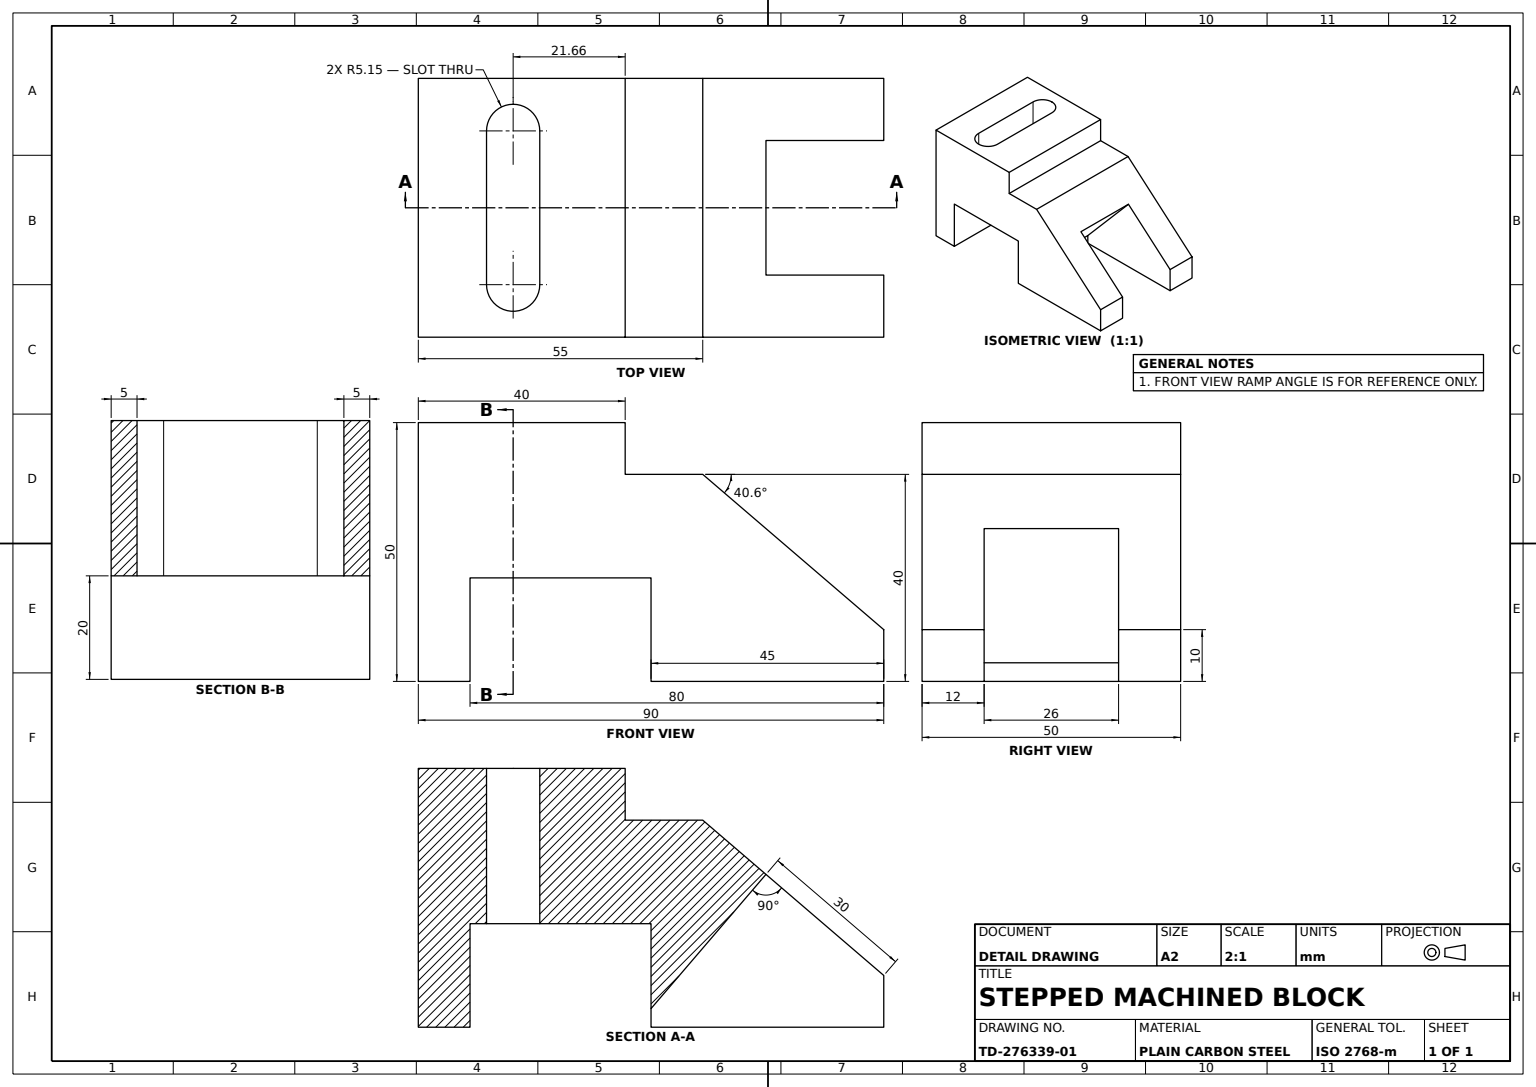
SolidWorks part; units mm, degrees
material "Plain Carbon Steel"
ref_plane "Front Plane" through (0, 0, 0) normal (0, 0, 1) x (1, 0, 0)
ref_plane "Top Plane" through (0, 0, 0) normal (0, 1, 0) x (1, 0, 0)
ref_plane "Right Plane" through (0, 0, 0) normal (1, 0, 0) x (0, 0, -1)
sketch "Support Profile Sketch" plane through (0, 0, 0) normal (0, 0, 1) x (1, 0, 0)
  line L0 (0, 0) -> (45, 0)
  line L1 (45, 0) -> (45, 20)
  line L2 (45, 20) -> (80, 20)
  line L3 (80, 20) -> (80, 0)
  line L4 (80, 0) -> (90, 0)
  line L5 (90, 0) -> (90, 50)
  line L6 (90, 50) -> (50, 50)
  line L7 (50, 50) -> (50, 40)
  line L8 (50, 40) -> (35, 40)
  line L9 (0, 0) -> (0, 10)
  line L10 (0, 10) -> (35, 40)
  dimension "D1" = 45
  dimension "D2" = 10
  dimension "D3" = 40
  dimension "D4" = 40
  dimension "D5" = 55
  dimension "D6" = 50
  dimension "D7" = 90
  dimension "D8" = 20
  dimension "D9" = 80
extrude "Support Body 50mm" add sketch "Support Profile Sketch" along normal blind 50
sketch "Top Slot Sketch" plane through (0, 50, 0) normal (0, 1, 0) x (1, 0, 0)
  line L0 (71.6617, -10.1471) -> (71.6617, -39.8529) construction
  line L1 (76.8088, -10.1471) -> (76.8088, -39.8529)
  line L2 (66.5147, -10.1471) -> (66.5147, -39.8529)
  line L3 (90, 0) -> (50, 0) construction
  line L4 (90, -50) -> (50, -50) construction
  line L5 (50, -50) -> (50, 0) construction
  arc A0 (76.8088, -10.1471) -> (66.5147, -10.1471) centre (71.6617, -10.1471) ccw
  arc A1 (66.5147, -39.8529) -> (76.8088, -39.8529) centre (71.6617, -39.8529) ccw
  point P2 (71.6617, -25)
  point P7 (71.6617, -5)
  point P12 (71.6617, -45)
  dimension "D3" = 5.1471
  dimension "D1" = 5
  dimension "D2" = 5
  dimension "D4" = 21.6617
extrude "Top Slot 34mm Deep" cut sketch "Top Slot Sketch" against normal blind 34
sketch "Clevis Notch Sketch" plane through (-4.9412, 5.7647, 0) normal (-0.6508, 0.7593, 0) x (0.7593, 0.6508, 0)
  line L1 (6.5079, -12) -> (36.5079, -12)
  line L2 (6.5079, -12) -> (6.5079, -38)
  line L3 (6.5079, -38) -> (36.5079, -38)
  line L4 (36.5079, -12) -> (36.5079, -38)
  line L5 (6.5079, -12) -> (36.5079, -38) construction
  line L6 (6.5079, -38) -> (36.5079, -12) construction
  line L7 (6.5079, -50) -> (6.5079, 0) construction
  point P0 (6.5079, -25)
  dimension "D1" = 30
  dimension "D2" = 26
  dimension "D3" = 12
extrude "Clevis Notch" cut sketch "Clevis Notch Sketch" against normal through all
sketch "Side Relief Sketch" plane through (0, 0, 0) normal (-1, 0, 0) x (0, 0, 1)
  line L0 (12, 10) -> (12, 0)
  line L1 (12, 0) -> (38, 0)
  line L2 (38, 0) -> (38, 10)
  line L3 (38, 10) -> (12, 10)
extrude "Side Relief Cut 10mm" cut sketch "Side Relief Sketch" against normal blind 10
